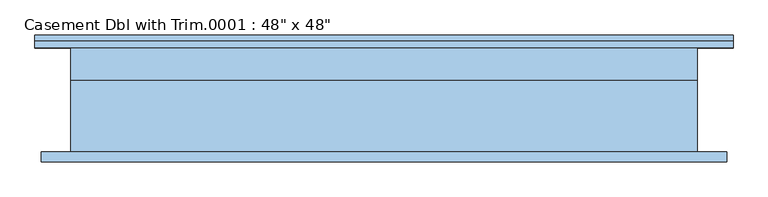
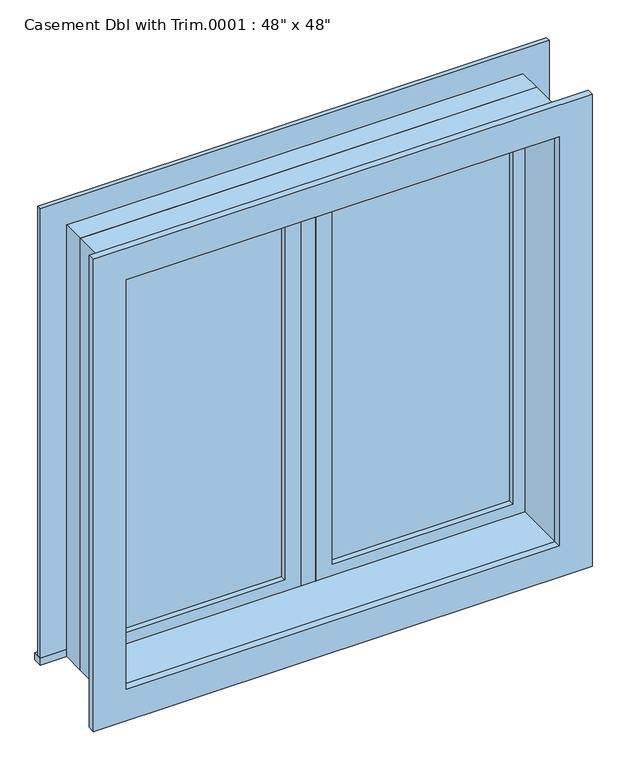
"""IFC4 building model written with IfcOpenShell, lengths in millimetres: window geometry."""

from ifc_helpers import new_model, si_unit, frame, origin, place, context, project, spatial, polyline, outline, extrude, source, transform, mapped, element, save


def window_0862ab64(model_context):
    return source(origin(), model_context, "Body", "SweptSolid", [
        extrude(outline(polyline([(63.5, 85.725), (546.1, 85.725), (546.1, 73.025), (63.5, 73.025), (63.5, 85.725)])), frame((0.0, 0.0, 977.9), z_axis=(0.0, 0.0, 1.0), x_axis=(1.0, 0.0, 0.0)), (0.0, 0.0, 1.0), 1092.2),
        extrude(outline(polyline([(2114.55, 19.05), (933.45, 19.05), (933.45, 590.55), (2114.55, 590.55), (2114.55, 19.05)]), holes=[polyline([(2070.1, 63.5), (2070.1, 546.1), (977.9, 546.1), (977.9, 63.5), (2070.1, 63.5)])]), frame((0.0, 57.15, 0.0), z_axis=(0.0, 1.0, 0.0), x_axis=(0.0, 0.0, 1.0)), (0.0, 0.0, 1.0), 44.45),
        extrude(outline(polyline([(19.05, 57.15), (-19.05, 57.15), (-19.05, 120.65), (19.05, 120.65), (19.05, 57.15)])), frame((0.0, 0.0, 933.45), z_axis=(0.0, 0.0, 1.0), x_axis=(1.0, 0.0, 0.0)), (0.0, 0.0, 1.0), 1181.1),
        extrude(outline(polyline([(-679.45, 146.05), (679.45, 146.05), (679.45, 120.65), (-679.45, 120.65), (-679.45, 146.05)])), frame((0.0, 0.0, 914.4), z_axis=(0.0, 0.0, 1.0), x_axis=(1.0, 0.0, 0.0)), (0.0, 0.0, 1.0), 19.05),
        extrude(outline(polyline([(2114.55, -590.55), (2114.55, 590.55), (933.45, 590.55), (933.45, 679.45), (2203.45, 679.45), (2203.45, -679.45), (933.45, -679.45), (933.45, -590.55), (2114.55, -590.55)])), frame((0.0, 120.65, 0.0), z_axis=(0.0, 1.0, 0.0), x_axis=(0.0, 0.0, 1.0)), (0.0, 0.0, 1.0), 12.7),
        extrude(outline(polyline([(2190.75, 666.75), (2190.75, -666.75), (857.25, -666.75), (857.25, 666.75), (2190.75, 666.75)]), holes=[polyline([(2101.85, 577.85), (946.15, 577.85), (946.15, -577.85), (2101.85, -577.85), (2101.85, 577.85)])]), frame((0.0, -101.6, 0.0), z_axis=(0.0, 1.0, 0.0), x_axis=(0.0, 0.0, 1.0)), (0.0, 0.0, 1.0), 19.05),
        extrude(outline(polyline([(-63.5, 73.025), (-546.1, 73.025), (-546.1, 85.725), (-63.5, 85.725), (-63.5, 73.025)])), frame((0.0, 0.0, 977.9), z_axis=(0.0, 0.0, 1.0), x_axis=(1.0, 0.0, 0.0)), (0.0, 0.0, 1.0), 1092.2),
        extrude(outline(polyline([(2114.55, -590.55), (933.45, -590.55), (933.45, -19.05), (2114.55, -19.05), (2114.55, -590.55)]), holes=[polyline([(2070.1, -546.1), (2070.1, -63.5), (977.9, -63.5), (977.9, -546.1), (2070.1, -546.1)])]), frame((0.0, 57.15, 0.0), z_axis=(0.0, 1.0, 0.0), x_axis=(0.0, 0.0, 1.0)), (0.0, 0.0, 1.0), 44.45),
        extrude(outline(polyline([(2133.6, -609.6), (914.4, -609.6), (914.4, 609.6), (2133.6, 609.6), (2133.6, -609.6)]), holes=[polyline([(2101.85, -577.85), (2101.85, 577.85), (946.15, 577.85), (946.15, -577.85), (2101.85, -577.85)])]), frame((0.0, -82.55, 0.0), z_axis=(0.0, 1.0, 0.0), x_axis=(0.0, 0.0, 1.0)), (0.0, 0.0, 1.0), 139.7),
        extrude(outline(polyline([(2133.6, 609.6), (2133.6, -609.6), (914.4, -609.6), (914.4, 609.6), (2133.6, 609.6)]), holes=[polyline([(2114.55, 590.55), (933.45, 590.55), (933.45, -590.55), (2114.55, -590.55), (2114.55, 590.55)])]), frame((0.0, 57.15, 0.0), z_axis=(0.0, 1.0, 0.0), x_axis=(0.0, 0.0, 1.0)), (0.0, 0.0, 1.0), 63.5),
    ])


if __name__ == "__main__":
    model = new_model("IFC4")
    model_context = context("Model", 3, world=origin())
    ifc_project = project(units=[si_unit("LENGTHUNIT", "METRE", prefix="MILLI")], contexts=[model_context])
    site = spatial("IfcSite", under=ifc_project)
    building = spatial("IfcBuilding", under=site)
    placement = place(None, origin())
    window_shape = window_0862ab64(model_context)
    element("IfcWindow", 1, ObjectType="Casement Dbl with Trim.0001 : 48\" x 48\"", at=placement, inside=building, context=model_context, shape_type="MappedRepresentation", body=[
        mapped(window_shape, transform((0.0, 0.0, 0.0), x_axis=(1.0, 0.0, 0.0), y_axis=(0.0, 1.0, 0.0), z_axis=(0.0, 0.0, 1.0))),
    ])
    save(model, "model.ifc")

# Revit data of these elements
# Type "Casement Dbl with Trim.0001 : 48\" x 48\""
#   Type Mark = "10"
#   Construction Type Id = "GSP4R"
#   Assembly Code = "B2020100"
#   Analytic Construction = "1/8 in Pilkington single glazing"
#   Visual Light Transmittance = 0.9
#   Solar Heat Gain Coefficient = 0.78
#   Heat Transfer Coefficient (U) = 0.6496 BTU/(h·ft²·°F)
#   Height = 4' - 0"
#   Default Sill Height = 3' - 0"
#   Trim Projection - Ext. = 0' - 0 1/2"
#   Trim Projection - Int. = 0' - 0 3/4"
#   Trim Width - Exterior = 0' - 3 1/2"
#   Trim Width - Interior = 0' - 3 1/2"
#   Width = 4' - 0"
#   Window Inset = 0' - 0 3/4"
#   Define Thermal Properties by = 1
#   Glass Pane Material = Glass
#   Sash Material = Sash
#   Trim Exterior Material = Trim
#   Trim Interior Material = Trim
#   Wall Closure = (empty or 0)
# Element 1 (IfcWindow, "Casement Dbl with Trim.0001 : 48\" x 48\"")
#   Materials on its faces: "Sash", "Trim", "Glass"
# Materials
#   "Glass": class "Glass", colour RGB 0 128 192, transparency 0.75, Description = "Soda Lime Glass", Cost = 0
#   "Sash": class "Wood", colour RGB 224 178 126, transparency 0
#   "Trim": class "Wood", colour RGB 224 178 126, transparency 0
